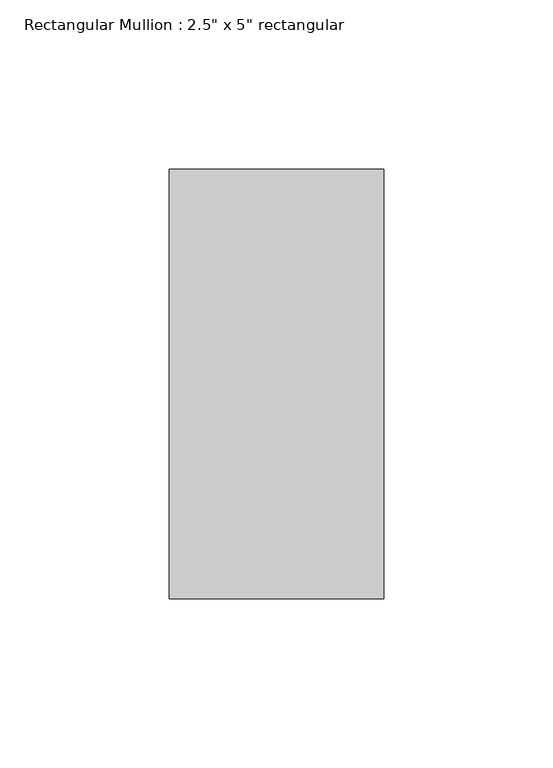
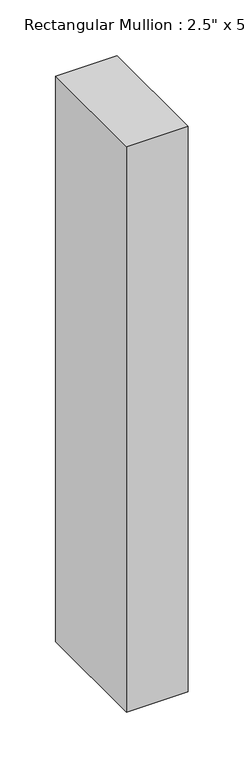
"""IFC4 building model written with IfcOpenShell, lengths in millimetres: member geometry."""

from ifc_helpers import new_model, si_unit, frame, origin, place, context, project, spatial, polyline, outline, extrude, source, transform, mapped, element, save


def member_01f21cfb(model_context):
    return source(origin(), model_context, "Body", "SweptSolid", [
        extrude(outline(polyline([(0.0, 63.5), (0.0, -63.5), (-63.5, -63.5), (-63.5, 63.5), (0.0, 63.5)])), frame((0.0, 0.0, -617.2348788), z_axis=(0.0, 0.0, 1.0), x_axis=(1.0, 0.0, 0.0)), (0.0, 0.0, 1.0), 617.2348788),
    ])


if __name__ == "__main__":
    model = new_model("IFC4")
    model_context = context("Model", 3, world=origin())
    ifc_project = project(units=[si_unit("LENGTHUNIT", "METRE", prefix="MILLI")], contexts=[model_context])
    site = spatial("IfcSite", under=ifc_project)
    building = spatial("IfcBuilding", under=site)
    placement = place(None, origin())
    member_shape = member_01f21cfb(model_context)
    element("IfcMember", 1, ObjectType="Rectangular Mullion : 2.5\" x 5\" rectangular", at=placement, inside=building, context=model_context, shape_type="MappedRepresentation", body=[
        mapped(member_shape, transform((0.0, 0.0, 0.0), x_axis=(1.0, 0.0, 0.0), y_axis=(0.0, 1.0, 0.0), z_axis=(0.0, 0.0, 1.0))),
    ])
    save(model, "model.ifc")

# Revit data of these elements
# Type "Rectangular Mullion : 2.5\" x 5\" rectangular"
#   built-in parameter 1007304 = 0.416667 (stored number, unit not read)
#   built-in parameter 1007301 = 0.104167 (stored number, unit not read)
#   built-in parameter 1007300 = 0.104167 (stored number, unit not read)
# Element 1 (IfcMember, "Rectangular Mullion : 2.5\" x 5\" rectangular")
#   Materials on its faces: "Aluminum"
# Materials
#   "Aluminum": class "Metal", colour RGB 247 247 247, transparency 0, Description = "Aluminum 6061", Cost = 0
